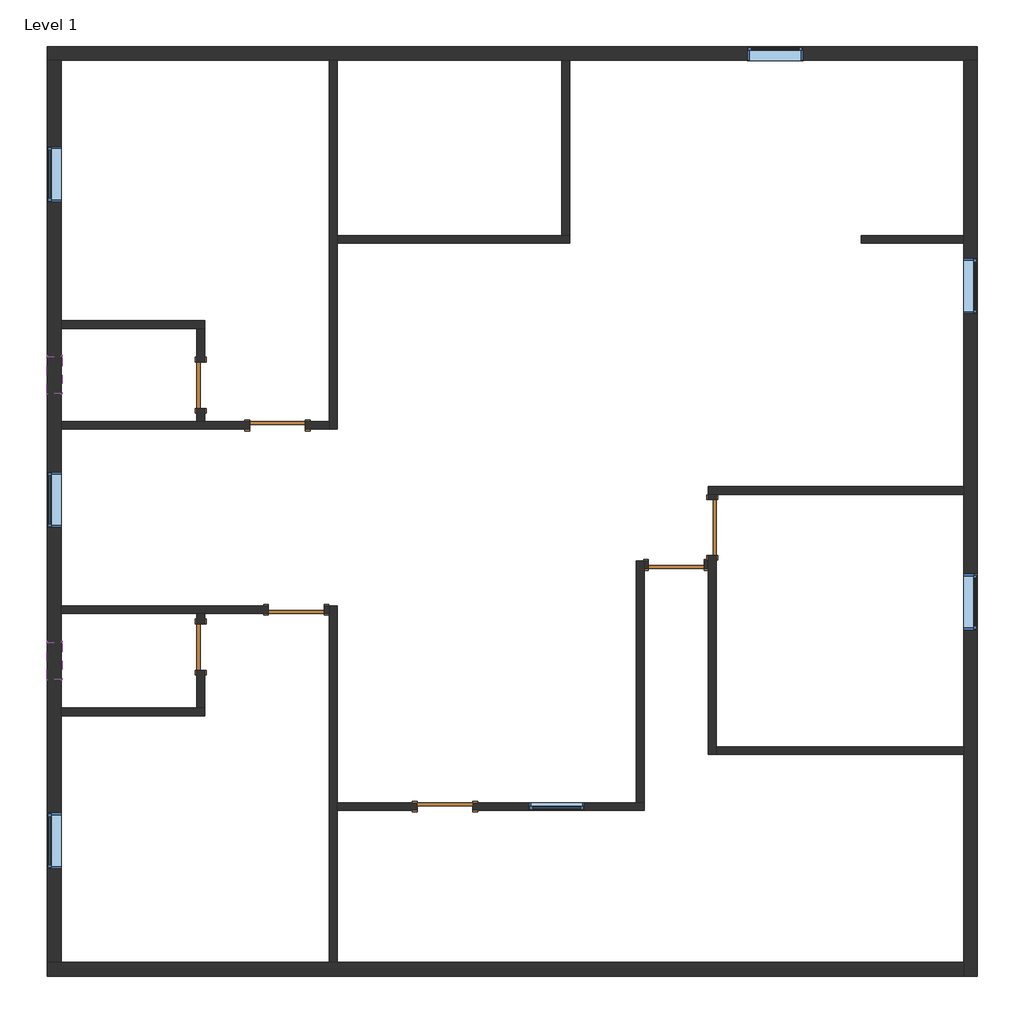
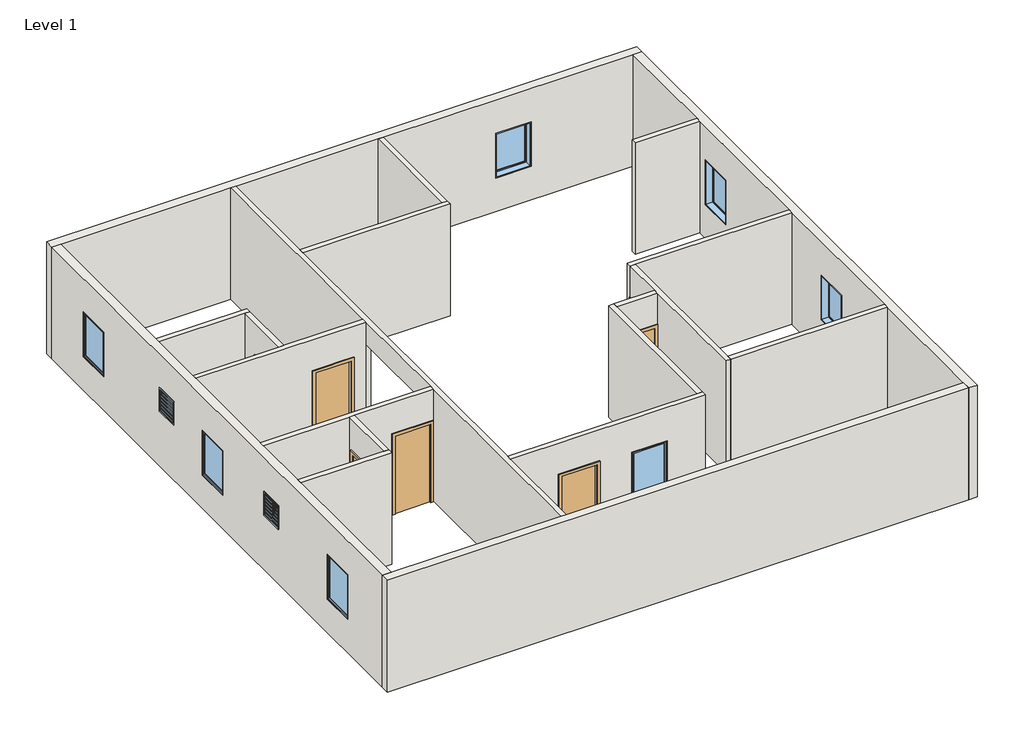
# One storey: 20 walls, 9 windows, 7 doors.
"""IFC4 building model written with IfcOpenShell, lengths in millimetres."""

from ifc_helpers import new_model, si_unit, frame, origin, origin_with_axes, place, context, project, spatial, polyline, outline, extrude, faceted_brep, transform, mapped, element, save
from components import door_4d6c7550, door_e36758a9, door_a1797ceb, door_a3eb833a, window_c1f32544, window_1bec9dad, window_f2d8fef0

model = new_model("IFC4")

# Units and contexts
model_context = context("Model", 3, world=origin())
ifc_project = project(units=[si_unit("LENGTHUNIT", "METRE", prefix="MILLI")], contexts=[model_context])

# Site, building, storey
site = spatial("IfcSite", under=ifc_project)
building = spatial("IfcBuilding", under=site)
storey = spatial("IfcBuildingStorey", under=building, Name="Level 1", Elevation=0.0)

# Doors
placement = place(None, origin())
door_shape = door_4d6c7550(model_context)
element("IfcDoor", 1, ObjectType="Single-Flush : 30\" x 84\"", at=placement, inside=storey, context=model_context, shape_type="MappedRepresentation", body=[
    mapped(door_shape, transform((-9496.7039913, -4083.9193327, 0.0), x_axis=(0.0, 1.0, 0.0), y_axis=(-1.0, 0.0, 0.0), z_axis=(0.0, 0.0, 1.0))),
])
door_2_shape = door_e36758a9(model_context)
element("IfcDoor", 2, ObjectType="Single-Flush : 30\" x 84\"", at=placement, inside=storey, context=model_context, shape_type="MappedRepresentation", body=[
    mapped(door_2_shape, transform((-9496.7039913, 208.6806673, 0.0), x_axis=(0.0, -1.0, 0.0), y_axis=(1.0, 0.0, 0.0), z_axis=(0.0, 0.0, 1.0))),
])
door_3_shape = door_a1797ceb(model_context)
element("IfcDoor", 3, ObjectType="Single-Flush : 36\" x 84\"", at=placement, inside=storey, context=model_context, shape_type="MappedRepresentation", body=[
    mapped(door_3_shape, transform((-8239.4039913, -451.7193327, 0.0), x_axis=(1.0, 0.0, 0.0), y_axis=(0.0, 1.0, 0.0), z_axis=(0.0, 0.0, 1.0))),
])
element("IfcDoor", 4, ObjectType="Single-Flush : 36\" x 84\"", at=placement, inside=storey, context=model_context, shape_type="MappedRepresentation", body=[
    mapped(door_3_shape, transform((-7934.6039913, -3474.3193327, 0.0), x_axis=(-1.0, 0.0, 0.0), y_axis=(0.0, -1.0, 0.0), z_axis=(0.0, 0.0, 1.0))),
])
element("IfcDoor", 5, ObjectType="Single-Flush : 36\" x 84\"", at=placement, inside=storey, context=model_context, shape_type="MappedRepresentation", body=[
    mapped(door_3_shape, transform((-1705.2539913, -2737.7193327, 0.0), x_axis=(-1.0, 0.0, 0.0), y_axis=(0.0, -1.0, 0.0), z_axis=(0.0, 0.0, 1.0))),
])
door_4_shape = door_a3eb833a(model_context)
element("IfcDoor", 6, ObjectType="Single-Flush : 36\" x 84\"", at=placement, inside=storey, context=model_context, shape_type="MappedRepresentation", body=[
    mapped(door_4_shape, transform((-1114.7039913, -2128.1193327, 0.0), x_axis=(0.0, 1.0, 0.0), y_axis=(-1.0, 0.0, 0.0), z_axis=(0.0, 0.0, 1.0))),
])
element("IfcDoor", 7, ObjectType="Single-Flush : 36\" x 84\"", at=placement, inside=storey, context=model_context, shape_type="MappedRepresentation", body=[
    mapped(door_4_shape, transform((-5496.2039913, -6700.1193327, 0.0), x_axis=(-1.0, 0.0, 0.0), y_axis=(0.0, -1.0, 0.0), z_axis=(0.0, 0.0, 1.0))),
])

# Walls
element("IfcWall", 8, ObjectType="Generic - 5\"", at=placement, inside=storey, context=model_context, shape_type="Brep", body=[
    faceted_brep([(-7261.5039913, 5529.9806673, 0.0), (-7261.5039913, 5529.9806673, 3048.0), (-7261.5039913, 2659.7806673, 3048.0), (-7261.5039913, 2532.7806673, 3048.0), (-7261.5039913, -6636.6193327, 3048.0), (-7261.5039913, -6763.6193327, 3048.0), (-7261.5039913, -9252.8193327, 3048.0), (-7261.5039913, -9252.8193327, 0.0), (-7261.5039913, -6763.6193327, 0.0), (-7261.5039913, -6636.6193327, 0.0), (-7261.5039913, -3410.8193327, 0.0), (-7261.5039913, -3410.8193327, 2438.4), (-7261.5039913, -515.2193327, 2438.4), (-7261.5039913, -515.2193327, 0.0), (-7261.5039913, 2532.7806673, 0.0), (-7261.5039913, 2659.7806673, 0.0), (-7388.5039913, 5529.9806673, 3048.0), (-7388.5039913, 5529.9806673, 0.0), (-7388.5039913, -388.2193327, 0.0), (-7388.5039913, -515.2193327, 0.0), (-7388.5039913, -515.2193327, 2438.4), (-7388.5039913, -3410.8193327, 2438.4), (-7388.5039913, -3410.8193327, 0.0), (-7388.5039913, -3537.8193327, 0.0), (-7388.5039913, -9252.8193327, 0.0), (-7388.5039913, -9252.8193327, 3048.0), (-7388.5039913, -3537.8193327, 3048.0), (-7388.5039913, -3410.8193327, 3048.0), (-7388.5039913, -515.2193327, 3048.0), (-7388.5039913, -388.2193327, 3048.0)], [[[0, 1, 2, 3, 4, 5, 6, 7, 8, 9, 10, 11, 12, 13, 14, 15]], [[16, 17, 18, 19, 20, 21, 22, 23, 24, 25, 26, 27, 28, 29]], [[7, 24, 23, 22, 10, 9, 8]], [[17, 0, 15, 14, 13, 19, 18]], [[6, 5, 4, 3, 2, 1, 16, 29, 28, 27, 26, 25]], [[7, 6, 25, 24]], [[1, 0, 17, 16]], [[11, 21, 20, 12]], [[21, 11, 10, 22]], [[12, 20, 19, 13]]]),
])
element("IfcWall", 9, ObjectType="Generic - 5\"", at=placement, inside=storey, context=model_context, shape_type="Brep", body=[
    faceted_brep([(-7261.5039913, 2532.7806673, 0.0), (-3451.5039913, 2532.7806673, 0.0), (-3451.5039913, 2532.7806673, 3048.0), (-7261.5039913, 2532.7806673, 3048.0), (-7261.5039913, 2659.7806673, 0.0), (-7261.5039913, 2659.7806673, 3048.0), (-3578.5039913, 2659.7806673, 3048.0), (-3451.5039913, 2659.7806673, 3048.0), (-3451.5039913, 2659.7806673, 0.0), (-3578.5039913, 2659.7806673, 0.0)], [[[0, 1, 2, 3]], [[4, 5, 6, 7, 8, 9]], [[1, 0, 4, 9, 8]], [[3, 2, 7, 6, 5]], [[0, 3, 5, 4]], [[2, 1, 8, 7]]]),
])
element("IfcWall", 10, ObjectType="Generic - 5\"", at=placement, inside=storey, context=model_context, shape_type="SweptSolid", body=[
    extrude(outline(polyline([(-3451.5039913, 5529.9806673), (-3451.5039913, 2659.7806673), (-3578.5039913, 2659.7806673), (-3578.5039913, 5529.9806673), (-3451.5039913, 5529.9806673)])), origin_with_axes(), (0.0, 0.0, 1.0), 3048.0),
])
element("IfcWall", 11, ObjectType="Generic - 5\"", at=placement, inside=storey, context=model_context, shape_type="SweptSolid", body=[
    extrude(outline(polyline([(1323.6960087, 2659.7806673), (3000.0960087, 2659.7806673), (3000.0960087, 2532.7806673), (1323.6960087, 2532.7806673), (1323.6960087, 2659.7806673)])), origin_with_axes(), (0.0, 0.0, 1.0), 3048.0),
])
element("IfcWall", 12, ObjectType="Generic - 5\"", at=placement, inside=storey, context=model_context, shape_type="SweptSolid", body=[
    extrude(outline(polyline([(0.0, -2232.3039913), (0.0, -2162.4539913), (2133.6, -2162.4539913), (2133.6, -1248.0539913), (0.0, -1248.0539913), (0.0, -1178.2039913), (3048.0, -1178.2039913), (3048.0, -2232.3039913), (0.0, -2232.3039913)])), frame((0.0, -2801.2193327, 0.0), z_axis=(0.0, 1.0, 0.0), x_axis=(0.0, 0.0, 1.0)), (0.0, 0.0, 1.0), 127.0),
])
element("IfcWall", 13, ObjectType="Generic - 5\"", at=placement, inside=storey, context=model_context, shape_type="Brep", body=[
    faceted_brep([(-1178.2039913, -1582.0193327, 0.0), (-1178.2039913, -1670.9193327, 0.0), (-1178.2039913, -1670.9193327, 2133.6), (-1178.2039913, -2585.3193327, 2133.6), (-1178.2039913, -2585.3193327, 0.0), (-1178.2039913, -2674.2193327, 0.0), (-1178.2039913, -2801.2193327, 0.0), (-1178.2039913, -5849.2193327, 0.0), (-1178.2039913, -5849.2193327, 3048.0), (-1178.2039913, -2801.2193327, 3048.0), (-1178.2039913, -2674.2193327, 3048.0), (-1178.2039913, -1582.0193327, 3048.0), (-1051.2039913, -1670.9193327, 2133.6), (-1051.2039913, -1670.9193327, 0.0), (-1051.2039913, -1582.0193327, 0.0), (-1051.2039913, -1582.0193327, 3048.0), (-1051.2039913, -5722.2193327, 3048.0), (-1051.2039913, -5849.2193327, 3048.0), (-1051.2039913, -5849.2193327, 0.0), (-1051.2039913, -5722.2193327, 0.0), (-1051.2039913, -2585.3193327, 0.0), (-1051.2039913, -2585.3193327, 2133.6)], [[[0, 1, 2, 3, 4, 5, 6, 7, 8, 9, 10, 11]], [[12, 13, 14, 15, 16, 17, 18, 19, 20, 21]], [[14, 13, 1, 0]], [[20, 19, 18, 7, 6, 5, 4]], [[11, 10, 9, 8, 17, 16, 15]], [[8, 7, 18, 17]], [[0, 11, 15, 14]], [[2, 1, 13, 12]], [[3, 2, 12, 21]], [[4, 3, 21, 20]]]),
])
element("IfcWall", 14, ObjectType="Generic - 5\"", at=placement, inside=storey, context=model_context, shape_type="SweptSolid", body=[
    extrude(outline(polyline([(3000.0960087, -5849.2193327), (-1051.2039913, -5849.2193327), (-1051.2039913, -5722.2193327), (3000.0960087, -5722.2193327), (3000.0960087, -5849.2193327)])), origin_with_axes(), (0.0, 0.0, 1.0), 3048.0),
])
element("IfcWall", 15, ObjectType="Generic - 5\"", at=placement, inside=storey, context=model_context, shape_type="Brep", body=[
    faceted_brep([(-7261.5039913, -6763.6193327, 0.0), (-5953.4039913, -6763.6193327, 0.0), (-5953.4039913, -6763.6193327, 2133.6), (-5039.0039913, -6763.6193327, 2133.6), (-5039.0039913, -6763.6193327, 0.0), (-2232.3039913, -6763.6193327, 0.0), (-2232.3039913, -6763.6193327, 3048.0), (-7261.5039913, -6763.6193327, 3048.0), (-4124.6039913, -6763.6193327, 2133.6), (-3210.2039913, -6763.6193327, 2133.6), (-3210.2039913, -6763.6193327, 914.4), (-4124.6039913, -6763.6193327, 914.4), (-5953.4039913, -6636.6193327, 2133.6), (-5953.4039913, -6636.6193327, 0.0), (-7261.5039913, -6636.6193327, 0.0), (-7261.5039913, -6636.6193327, 3048.0), (-2359.3039913, -6636.6193327, 3048.0), (-2232.3039913, -6636.6193327, 3048.0), (-2232.3039913, -6636.6193327, 0.0), (-2359.3039913, -6636.6193327, 0.0), (-5039.0039913, -6636.6193327, 0.0), (-5039.0039913, -6636.6193327, 2133.6), (-4124.6039913, -6636.6193327, 2133.6), (-4124.6039913, -6636.6193327, 914.4), (-3210.2039913, -6636.6193327, 914.4), (-3210.2039913, -6636.6193327, 2133.6)], [[[0, 1, 2, 3, 4, 5, 6, 7], [8, 9, 10, 11]], [[12, 13, 14, 15, 16, 17, 18, 19, 20, 21], [22, 23, 24, 25]], [[14, 13, 1, 0]], [[20, 19, 18, 5, 4]], [[7, 6, 17, 16, 15]], [[0, 7, 15, 14]], [[6, 5, 18, 17]], [[2, 1, 13, 12]], [[3, 2, 12, 21]], [[4, 3, 21, 20]], [[23, 22, 8, 11]], [[24, 23, 11, 10]], [[25, 24, 10, 9]], [[22, 25, 9, 8]]]),
])
element("IfcWall", 16, ObjectType="Generic - 5\"", at=placement, inside=storey, context=model_context, shape_type="Brep", body=[
    faceted_brep([(-2232.3039913, -6636.6193327, 0.0), (-2232.3039913, -2801.2193327, 0.0), (-2232.3039913, -2674.2193327, 0.0), (-2232.3039913, -2674.2193327, 3048.0), (-2232.3039913, -2801.2193327, 3048.0), (-2232.3039913, -6636.6193327, 3048.0), (-2359.3039913, -6636.6193327, 0.0), (-2359.3039913, -6636.6193327, 3048.0), (-2359.3039913, -2674.2193327, 3048.0), (-2359.3039913, -2674.2193327, 0.0)], [[[0, 1, 2, 3, 4, 5]], [[6, 7, 8, 9]], [[2, 1, 0, 6, 9]], [[5, 4, 3, 8, 7]], [[0, 5, 7, 6]], [[3, 2, 9, 8]]]),
])
element("IfcWall", 17, ObjectType="Generic - 5\"", at=placement, inside=storey, context=model_context, shape_type="Brep", body=[
    faceted_brep([(-11782.7039913, -5214.2193327, 0.0), (-9433.2039913, -5214.2193327, 0.0), (-9433.2039913, -5214.2193327, 3048.0), (-11782.7039913, -5214.2193327, 3048.0), (-11782.7039913, -5087.2193327, 0.0), (-11782.7039913, -5087.2193327, 3048.0), (-9560.2039913, -5087.2193327, 3048.0), (-9433.2039913, -5087.2193327, 3048.0), (-9433.2039913, -5087.2193327, 0.0), (-9560.2039913, -5087.2193327, 0.0)], [[[0, 1, 2, 3]], [[4, 5, 6, 7, 8, 9]], [[1, 0, 4, 9, 8]], [[3, 2, 7, 6, 5]], [[0, 3, 5, 4]], [[2, 1, 8, 7]]]),
])
element("IfcWall", 18, ObjectType="Generic - 5\"", at=placement, inside=storey, context=model_context, shape_type="SweptSolid", body=[
    extrude(outline(polyline([(-3537.8193327, 0.0), (-3702.9193327, 0.0), (-3702.9193327, 2133.6), (-4464.9193327, 2133.6), (-4464.9193327, 0.0), (-5087.2193327, 0.0), (-5087.2193327, 3048.0), (-3537.8193327, 3048.0), (-3537.8193327, 0.0)])), frame((-9560.2039913, 0.0, 0.0), z_axis=(1.0, 0.0, 0.0), x_axis=(0.0, 1.0, 0.0)), (0.0, 0.0, 1.0), 127.0),
])
element("IfcWall", 19, ObjectType="Generic - 5\"", at=placement, inside=storey, context=model_context, shape_type="Brep", body=[
    faceted_brep([(-8391.8039913, -3410.8193327, 2133.6), (-8391.8039913, -3410.8193327, 0.0), (-11782.7039913, -3410.8193327, 0.0), (-11782.7039913, -3410.8193327, 3048.0), (-7388.5039913, -3410.8193327, 3048.0), (-7388.5039913, -3410.8193327, 2438.4), (-7388.5039913, -3410.8193327, 0.0), (-7477.4039913, -3410.8193327, 0.0), (-7477.4039913, -3410.8193327, 2133.6), (-11782.7039913, -3537.8193327, 0.0), (-9560.2039913, -3537.8193327, 0.0), (-9433.2039913, -3537.8193327, 0.0), (-8391.8039913, -3537.8193327, 0.0), (-8391.8039913, -3537.8193327, 2133.6), (-7477.4039913, -3537.8193327, 2133.6), (-7477.4039913, -3537.8193327, 0.0), (-7388.5039913, -3537.8193327, 0.0), (-7388.5039913, -3537.8193327, 3048.0), (-9433.2039913, -3537.8193327, 3048.0), (-9560.2039913, -3537.8193327, 3048.0), (-11782.7039913, -3537.8193327, 3048.0)], [[[0, 1, 2, 3, 4, 5, 6, 7, 8]], [[9, 10, 11, 12, 13, 14, 15, 16, 17, 18, 19, 20]], [[7, 6, 16, 15]], [[2, 1, 12, 11, 10, 9]], [[4, 3, 20, 19, 18, 17]], [[3, 2, 9, 20]], [[6, 5, 4, 17, 16]], [[13, 12, 1, 0]], [[14, 13, 0, 8]], [[15, 14, 8, 7]]]),
])
element("IfcWall", 20, ObjectType="Generic - 5\"", at=placement, inside=storey, context=model_context, shape_type="Brep", body=[
    faceted_brep([(-7388.5039913, -388.2193327, 0.0), (-7782.2039913, -388.2193327, 0.0), (-7782.2039913, -388.2193327, 2133.6), (-8696.6039913, -388.2193327, 2133.6), (-8696.6039913, -388.2193327, 0.0), (-9433.2039913, -388.2193327, 0.0), (-9560.2039913, -388.2193327, 0.0), (-11782.7039913, -388.2193327, 0.0), (-11782.7039913, -388.2193327, 3048.0), (-9560.2039913, -388.2193327, 3048.0), (-9433.2039913, -388.2193327, 3048.0), (-7388.5039913, -388.2193327, 3048.0), (-7782.2039913, -515.2193327, 2133.6), (-7782.2039913, -515.2193327, 0.0), (-7388.5039913, -515.2193327, 0.0), (-7388.5039913, -515.2193327, 2438.4), (-7388.5039913, -515.2193327, 3048.0), (-11782.7039913, -515.2193327, 3048.0), (-11782.7039913, -515.2193327, 0.0), (-8696.6039913, -515.2193327, 0.0), (-8696.6039913, -515.2193327, 2133.6)], [[[0, 1, 2, 3, 4, 5, 6, 7, 8, 9, 10, 11]], [[12, 13, 14, 15, 16, 17, 18, 19, 20]], [[19, 18, 7, 6, 5, 4]], [[14, 13, 1, 0]], [[11, 10, 9, 8, 17, 16]], [[8, 7, 18, 17]], [[0, 11, 16, 15, 14]], [[2, 1, 13, 12]], [[3, 2, 12, 20]], [[4, 3, 20, 19]]]),
])
element("IfcWall", 21, ObjectType="Generic - 5\"", at=placement, inside=storey, context=model_context, shape_type="Brep", body=[
    faceted_brep([(-9433.2039913, 1262.7806673, 0.0), (-11782.7039913, 1262.7806673, 0.0), (-11782.7039913, 1262.7806673, 3048.0), (-9433.2039913, 1262.7806673, 3048.0), (-9433.2039913, 1135.7806673, 0.0), (-9433.2039913, 1135.7806673, 3048.0), (-9560.2039913, 1135.7806673, 3048.0), (-11782.7039913, 1135.7806673, 3048.0), (-11782.7039913, 1135.7806673, 0.0), (-9560.2039913, 1135.7806673, 0.0)], [[[0, 1, 2, 3]], [[4, 5, 6, 7, 8, 9]], [[1, 0, 4, 9, 8]], [[3, 2, 7, 6, 5]], [[2, 1, 8, 7]], [[0, 3, 5, 4]]]),
])
element("IfcWall", 22, ObjectType="Generic - 5\"", at=placement, inside=storey, context=model_context, shape_type="SweptSolid", body=[
    extrude(outline(polyline([(-172.3193327, 2133.6), (-172.3193327, 0.0), (-388.2193327, 0.0), (-388.2193327, 3048.0), (1135.7806673, 3048.0), (1135.7806673, 0.0), (589.6806673, 0.0), (589.6806673, 2133.6), (-172.3193327, 2133.6)])), frame((-9560.2039913, 0.0, 0.0), z_axis=(1.0, 0.0, 0.0), x_axis=(0.0, 1.0, 0.0)), (0.0, 0.0, 1.0), 127.0),
])
element("IfcWall", 23, ObjectType="Generic - 5\"", at=placement, inside=storey, context=model_context, shape_type="Brep", body=[
    faceted_brep([(3000.0960087, -1455.0193327, 0.0), (-1178.2039913, -1455.0193327, 0.0), (-1178.2039913, -1455.0193327, 3048.0), (3000.0960087, -1455.0193327, 3048.0), (3000.0960087, -1582.0193327, 0.0), (3000.0960087, -1582.0193327, 3048.0), (-1051.2039913, -1582.0193327, 3048.0), (-1178.2039913, -1582.0193327, 3048.0), (-1178.2039913, -1582.0193327, 0.0), (-1051.2039913, -1582.0193327, 0.0)], [[[0, 1, 2, 3]], [[4, 5, 6, 7, 8, 9]], [[1, 0, 4, 9, 8]], [[3, 2, 7, 6, 5]], [[0, 3, 5, 4]], [[2, 1, 8, 7]]]),
])
element("IfcWall", 24, ObjectType="Generic - 9\"", at=placement, inside=storey, context=model_context, shape_type="Brep", body=[
    faceted_brep([(-12011.3039913, 5529.9806673, 0.0), (-11782.7039913, 5529.9806673, 0.0), (-7388.5039913, 5529.9806673, 0.0), (-7261.5039913, 5529.9806673, 0.0), (-3578.5039913, 5529.9806673, 0.0), (-3451.5039913, 5529.9806673, 0.0), (3000.0960087, 5529.9806673, 0.0), (3228.6960087, 5529.9806673, 0.0), (3228.6960087, 5529.9806673, 3048.0), (3000.0960087, 5529.9806673, 3048.0), (-3451.5039913, 5529.9806673, 3048.0), (-3578.5039913, 5529.9806673, 3048.0), (-7261.5039913, 5529.9806673, 3048.0), (-7388.5039913, 5529.9806673, 3048.0), (-11782.7039913, 5529.9806673, 3048.0), (-12011.3039913, 5529.9806673, 3048.0), (371.1960087, 5529.9806673, 2133.6), (371.1960087, 5529.9806673, 914.4), (-543.2039913, 5529.9806673, 914.4), (-543.2039913, 5529.9806673, 2133.6), (-12011.3039913, 5758.5806673, 0.0), (-12011.3039913, 5758.5806673, 3048.0), (3228.6960087, 5758.5806673, 3048.0), (3228.6960087, 5758.5806673, 0.0), (371.1960087, 5758.5806673, 2133.6), (-543.2039913, 5758.5806673, 2133.6), (-543.2039913, 5758.5806673, 914.4), (371.1960087, 5758.5806673, 914.4)], [[[0, 1, 2, 3, 4, 5, 6, 7, 8, 9, 10, 11, 12, 13, 14, 15], [16, 17, 18, 19]], [[20, 21, 22, 23], [24, 25, 26, 27]], [[7, 6, 5, 4, 3, 2, 1, 0, 20, 23]], [[15, 14, 13, 12, 11, 10, 9, 8, 22, 21]], [[8, 7, 23, 22]], [[0, 15, 21, 20]], [[17, 16, 24, 27]], [[18, 17, 27, 26]], [[19, 18, 26, 25]], [[16, 19, 25, 24]]]),
])
element("IfcWall", 25, ObjectType="Generic - 9\"", at=placement, inside=storey, context=model_context, shape_type="Brep", body=[
    faceted_brep([(3000.0960087, 5529.9806673, 0.0), (3000.0960087, 2659.7806673, 0.0), (3000.0960087, 2532.7806673, 0.0), (3000.0960087, -1455.0193327, 0.0), (3000.0960087, -1582.0193327, 0.0), (3000.0960087, -5722.2193327, 0.0), (3000.0960087, -5849.2193327, 0.0), (3000.0960087, -9252.8193327, 0.0), (3000.0960087, -9481.4193327, 0.0), (3000.0960087, -9481.4193327, 3048.0), (3000.0960087, -9252.8193327, 3048.0), (3000.0960087, -5849.2193327, 3048.0), (3000.0960087, -5722.2193327, 3048.0), (3000.0960087, -1582.0193327, 3048.0), (3000.0960087, -1455.0193327, 3048.0), (3000.0960087, 2532.7806673, 3048.0), (3000.0960087, 2659.7806673, 3048.0), (3000.0960087, 5529.9806673, 3048.0), (3000.0960087, -3804.5193327, 2133.6), (3000.0960087, -3804.5193327, 914.4), (3000.0960087, -2890.1193327, 914.4), (3000.0960087, -2890.1193327, 2133.6), (3000.0960087, 1377.0806673, 2133.6), (3000.0960087, 1377.0806673, 914.4), (3000.0960087, 2291.4806673, 914.4), (3000.0960087, 2291.4806673, 2133.6), (3228.6960087, 5529.9806673, 0.0), (3228.6960087, 5529.9806673, 3048.0), (3228.6960087, -9481.4193327, 3048.0), (3228.6960087, -9481.4193327, 0.0), (3228.6960087, -3804.5193327, 2133.6), (3228.6960087, -2890.1193327, 2133.6), (3228.6960087, -2890.1193327, 914.4), (3228.6960087, -3804.5193327, 914.4), (3228.6960087, 1377.0806673, 2133.6), (3228.6960087, 2291.4806673, 2133.6), (3228.6960087, 2291.4806673, 914.4), (3228.6960087, 1377.0806673, 914.4)], [[[0, 1, 2, 3, 4, 5, 6, 7, 8, 9, 10, 11, 12, 13, 14, 15, 16, 17], [18, 19, 20, 21], [22, 23, 24, 25]], [[26, 27, 28, 29], [30, 31, 32, 33], [34, 35, 36, 37]], [[8, 7, 6, 5, 4, 3, 2, 1, 0, 26, 29]], [[17, 16, 15, 14, 13, 12, 11, 10, 9, 28, 27]], [[0, 17, 27, 26]], [[9, 8, 29, 28]], [[19, 18, 30, 33]], [[20, 19, 33, 32]], [[21, 20, 32, 31]], [[18, 21, 31, 30]], [[23, 22, 34, 37]], [[24, 23, 37, 36]], [[25, 24, 36, 35]], [[22, 25, 35, 34]]]),
])
element("IfcWall", 26, ObjectType="Generic - 9\"", at=placement, inside=storey, context=model_context, shape_type="Brep", body=[
    faceted_brep([(3000.0960087, -9252.8193327, 0.0), (-7261.5039913, -9252.8193327, 0.0), (-7388.5039913, -9252.8193327, 0.0), (-11782.7039913, -9252.8193327, 0.0), (-12011.3039913, -9252.8193327, 0.0), (-12011.3039913, -9252.8193327, 3048.0), (-11782.7039913, -9252.8193327, 3048.0), (-7388.5039913, -9252.8193327, 3048.0), (-7261.5039913, -9252.8193327, 3048.0), (3000.0960087, -9252.8193327, 3048.0), (3000.0960087, -9481.4193327, 0.0), (3000.0960087, -9481.4193327, 3048.0), (-12011.3039913, -9481.4193327, 3048.0), (-12011.3039913, -9481.4193327, 0.0)], [[[0, 1, 2, 3, 4, 5, 6, 7, 8, 9]], [[10, 11, 12, 13]], [[4, 3, 2, 1, 0, 10, 13]], [[9, 8, 7, 6, 5, 12, 11]], [[0, 9, 11, 10]], [[5, 4, 13, 12]]]),
])
element("IfcWall", 27, ObjectType="Generic - 9\"", at=placement, inside=storey, context=model_context, shape_type="Brep", body=[
    faceted_brep([(-11782.7039913, -9252.8193327, 0.0), (-11782.7039913, -5214.2193327, 0.0), (-11782.7039913, -5087.2193327, 0.0), (-11782.7039913, -3537.8193327, 0.0), (-11782.7039913, -3410.8193327, 0.0), (-11782.7039913, -515.2193327, 0.0), (-11782.7039913, -388.2193327, 0.0), (-11782.7039913, 1135.7806673, 0.0), (-11782.7039913, 1262.7806673, 0.0), (-11782.7039913, 5529.9806673, 0.0), (-11782.7039913, 5529.9806673, 3048.0), (-11782.7039913, 1262.7806673, 3048.0), (-11782.7039913, 1135.7806673, 3048.0), (-11782.7039913, -388.2193327, 3048.0), (-11782.7039913, -515.2193327, 3048.0), (-11782.7039913, -3410.8193327, 3048.0), (-11782.7039913, -3537.8193327, 3048.0), (-11782.7039913, -5087.2193327, 3048.0), (-11782.7039913, -5214.2193327, 3048.0), (-11782.7039913, -9252.8193327, 3048.0), (-11782.7039913, 4120.2806673, 2133.6), (-11782.7039913, 4120.2806673, 914.4), (-11782.7039913, 3205.8806673, 914.4), (-11782.7039913, 3205.8806673, 2133.6), (-11782.7039913, -6801.7193327, 2133.6), (-11782.7039913, -6801.7193327, 914.4), (-11782.7039913, -7716.1193327, 914.4), (-11782.7039913, -7716.1193327, 2133.6), (-11782.7039913, -1213.7193327, 2133.6), (-11782.7039913, -1213.7193327, 914.4), (-11782.7039913, -2128.1193327, 914.4), (-11782.7039913, -2128.1193327, 2133.6), (-11782.7039913, 68.9806673, 2133.6), (-11782.7039913, 678.5806673, 2133.6), (-11782.7039913, 678.5806673, 1524.0), (-11782.7039913, 68.9806673, 1524.0), (-11782.7039913, -4617.3193327, 2133.6), (-11782.7039913, -4007.7193327, 2133.6), (-11782.7039913, -4007.7193327, 1524.0), (-11782.7039913, -4617.3193327, 1524.0), (-12011.3039913, -9252.8193327, 0.0), (-12011.3039913, -9252.8193327, 3048.0), (-12011.3039913, 5529.9806673, 3048.0), (-12011.3039913, 5529.9806673, 0.0), (-12011.3039913, 4120.2806673, 2133.6), (-12011.3039913, 3205.8806673, 2133.6), (-12011.3039913, 3205.8806673, 914.4), (-12011.3039913, 4120.2806673, 914.4), (-12011.3039913, -6801.7193327, 2133.6), (-12011.3039913, -7716.1193327, 2133.6), (-12011.3039913, -7716.1193327, 914.4), (-12011.3039913, -6801.7193327, 914.4), (-12011.3039913, -1213.7193327, 2133.6), (-12011.3039913, -2128.1193327, 2133.6), (-12011.3039913, -2128.1193327, 914.4), (-12011.3039913, -1213.7193327, 914.4), (-12011.3039913, 68.9806673, 2133.6), (-12011.3039913, 68.9806673, 1524.0), (-12011.3039913, 678.5806673, 1524.0), (-12011.3039913, 678.5806673, 2133.6), (-12011.3039913, -4617.3193327, 2133.6), (-12011.3039913, -4617.3193327, 1524.0), (-12011.3039913, -4007.7193327, 1524.0), (-12011.3039913, -4007.7193327, 2133.6)], [[[0, 1, 2, 3, 4, 5, 6, 7, 8, 9, 10, 11, 12, 13, 14, 15, 16, 17, 18, 19], [20, 21, 22, 23], [24, 25, 26, 27], [28, 29, 30, 31], [32, 33, 34, 35], [36, 37, 38, 39]], [[40, 41, 42, 43], [44, 45, 46, 47], [48, 49, 50, 51], [52, 53, 54, 55], [56, 57, 58, 59], [60, 61, 62, 63]], [[9, 8, 7, 6, 5, 4, 3, 2, 1, 0, 40, 43]], [[19, 18, 17, 16, 15, 14, 13, 12, 11, 10, 42, 41]], [[0, 19, 41, 40]], [[10, 9, 43, 42]], [[21, 20, 44, 47]], [[22, 21, 47, 46]], [[23, 22, 46, 45]], [[20, 23, 45, 44]], [[25, 24, 48, 51]], [[26, 25, 51, 50]], [[27, 26, 50, 49]], [[24, 27, 49, 48]], [[29, 28, 52, 55]], [[30, 29, 55, 54]], [[31, 30, 54, 53]], [[28, 31, 53, 52]], [[57, 56, 32, 35]], [[58, 57, 35, 34]], [[59, 58, 34, 33]], [[56, 59, 33, 32]], [[61, 60, 36, 39]], [[62, 61, 39, 38]], [[63, 62, 38, 37]], [[60, 63, 37, 36]]]),
])

# Windows
window_shape = window_c1f32544(model_context)
element("IfcWindow", 28, ObjectType="Fixed : 36\" x 48\"", at=placement, inside=storey, context=model_context, shape_type="MappedRepresentation", body=[
    mapped(window_shape, transform((-11897.0039913, 3701.1806673, 0.0), x_axis=(0.0, 1.0, 0.0), y_axis=(-1.0, 0.0, 0.0), z_axis=(0.0, 0.0, 1.0))),
])
element("IfcWindow", 29, ObjectType="Fixed : 36\" x 48\"", at=placement, inside=storey, context=model_context, shape_type="MappedRepresentation", body=[
    mapped(window_shape, transform((-11897.0039913, -7220.8193327, 0.0), x_axis=(0.0, 1.0, 0.0), y_axis=(-1.0, 0.0, 0.0), z_axis=(0.0, 0.0, 1.0))),
])
element("IfcWindow", 30, ObjectType="Fixed : 36\" x 48\"", at=placement, inside=storey, context=model_context, shape_type="MappedRepresentation", body=[
    mapped(window_shape, transform((3114.3960087, -3385.4193327, 0.0), x_axis=(0.0, -1.0, 0.0), y_axis=(1.0, 0.0, 0.0), z_axis=(0.0, 0.0, 1.0))),
])
element("IfcWindow", 31, ObjectType="Fixed : 36\" x 48\"", at=placement, inside=storey, context=model_context, shape_type="MappedRepresentation", body=[
    mapped(window_shape, transform((3114.3960087, 1796.1806673, 0.0), x_axis=(0.0, -1.0, 0.0), y_axis=(1.0, 0.0, 0.0), z_axis=(0.0, 0.0, 1.0))),
])
element("IfcWindow", 32, ObjectType="Fixed : 36\" x 48\"", at=placement, inside=storey, context=model_context, shape_type="MappedRepresentation", body=[
    mapped(window_shape, transform((-47.9039913, 5644.2806673, 0.0), x_axis=(1.0, 0.0, 0.0), y_axis=(0.0, 1.0, 0.0), z_axis=(0.0, 0.0, 1.0))),
])
element("IfcWindow", 33, ObjectType="Fixed : 36\" x 48\"", at=placement, inside=storey, context=model_context, shape_type="MappedRepresentation", body=[
    mapped(window_shape, transform((-11897.0039913, -1632.8193327, 0.0), x_axis=(0.0, 1.0, 0.0), y_axis=(-1.0, 0.0, 0.0), z_axis=(0.0, 0.0, 1.0))),
])
window_2_shape = window_1bec9dad(model_context)
element("IfcWindow", 34, ObjectType="Fixed : 36\" x 48\"", at=placement, inside=storey, context=model_context, shape_type="MappedRepresentation", body=[
    mapped(window_2_shape, transform((-3705.5039913, -6700.1193327, 0.0), x_axis=(-1.0, 0.0, 0.0), y_axis=(0.0, -1.0, 0.0), z_axis=(0.0, 0.0, 1.0))),
])
window_3_shape = window_f2d8fef0(model_context)
element("IfcWindow", 35, ObjectType="Window-Louvers : 24\" x 24\"", at=placement, inside=storey, context=model_context, shape_type="MappedRepresentation", body=[
    mapped(window_3_shape, transform((-11903.3539913, 373.7806673, 609.6), x_axis=(0.0, 1.0, 0.0), y_axis=(-1.0, 0.0, 0.0), z_axis=(0.0, 0.0, 1.0))),
])
element("IfcWindow", 36, ObjectType="Window-Louvers : 24\" x 24\"", at=placement, inside=storey, context=model_context, shape_type="MappedRepresentation", body=[
    mapped(window_3_shape, transform((-11903.3539913, -4312.5193327, 609.6), x_axis=(0.0, 1.0, 0.0), y_axis=(-1.0, 0.0, 0.0), z_axis=(0.0, 0.0, 1.0))),
])

save(model, "model.ifc")

# Revit data of these elements
# Type "Single-Flush : 30\" x 84\""
#   Type Mark = "4"
#   Construction Type Id = "MDOOR"
#   Assembly Code = "C1020"
#   Analytic Construction = "Metal"
#   Thickness = 0' - 2"
#   Heat Transfer Coefficient (U) = 0.651978 BTU/(h·ft²·°F)
#   Height = 7' - 0"
#   Trim Projection Ext = 0' - 1"
#   Trim Projection Int = 0' - 1"
#   Trim Width = 0' - 3"
#   Width = 2' - 6"
#   Define Thermal Properties by = 1
#   Define Thermal Properties by = 1
#   Door Material = Door - Panel
#   Frame Material = Door - Frame
#   Visual Light Transmittance = 0
#   Solar Heat Gain Coefficient = 0
#   Function = (empty or 0)
#   Wall Closure = (empty or 0)
# Type "Single-Flush : 36\" x 84\""
#   Type Mark = "1"
#   Construction Type Id = "MDOOR"
#   Assembly Code = "C1020"
#   Analytic Construction = "Metal"
#   Thickness = 0' - 2"
#   Heat Transfer Coefficient (U) = 0.651978 BTU/(h·ft²·°F)
#   Height = 7' - 0"
#   Trim Projection Ext = 0' - 1"
#   Trim Projection Int = 0' - 1"
#   Trim Width = 0' - 3"
#   Width = 3' - 0"
#   Define Thermal Properties by = 1
#   Define Thermal Properties by = 1
#   Door Material = Door - Panel
#   Frame Material = Door - Frame
#   Visual Light Transmittance = 0
#   Solar Heat Gain Coefficient = 0
#   Function = (empty or 0)
#   Wall Closure = (empty or 0)
# Type "Generic - 5\""
#   Assembly Code = "B2010"
#   Layers, outside or top first: 0' - 5" no material (function 1)
# Type "Generic - 9\""
#   Assembly Code = "B2010"
#   Layers, outside or top first: 0' - 9" no material (function 1)
# Type "Fixed : 36\" x 48\""
#   Type Mark = "W1"
#   Construction Type Id = "GSP4R"
#   Assembly Code = "B2020100"
#   Analytic Construction = "1/8 in Pilkington single glazing"
#   Visual Light Transmittance = 0.9
#   Solar Heat Gain Coefficient = 0.78
#   Heat Transfer Coefficient (U) = 0.6496 BTU/(h·ft²·°F)
#   Height = 4' - 0"
#   Default Sill Height = 3' - 0"
#   Width = 3' - 0"
#   Window Inset = 0' - 0 3/4"
#   Define Thermal Properties by = 1
#   Define Thermal Properties by = 1
#   Glass Pane Material = Glass
#   Sash Material = Sash
#   Wall Closure = (empty or 0)
# Type "Window-Louvers : 24\" x 24\""
#   Type Mark = "V1"
#   Construction Type Id = "GSP4R"
#   Assembly Code = "B20"
#   Analytic Construction = "1/8 in Pilkington single glazing"
#   Visual Light Transmittance = 0.9
#   Thermal Resistance (R) = 1.53941 (h·ft²·°F)/BTU
#   Solar Heat Gain Coefficient = 0.78
#   Max Height = 1' - 11.74264"
#   Height = 2' - 0"
#   Heat Transfer Coefficient (U) = 0.6496 BTU/(h·ft²·°F)
#   Blade Width [instance default] = 1' - 10 1/2"
#   Blade Vertical Thickness = 0' - 0.35355"
#   Blade Thickness = 0' - 0 1/4"
#   Blade Spacing = 0' - 1 1/2"
#   Blade Height = 0' - 1.85355"
#   Blade Depth = 0' - 3"
#   Blade Angle = 45.00°
#   Default Sill Height = 3' - 0"
#   Trim Projection_Exterior = 0' - 0 1/2"
#   Trim Projection_Interior = 0' - 0 1/2"
#   Trim Width_Exterior = 0' - 1 1/2"
#   Trim Width_Interior = 0' - 1 1/2"
#   Width = 2' - 0"
#   Max Blade Count = 12
#   Define Thermal Properties by = 1
#   Blade Count = 12
#   Frame Material = Birch
#   Louver Material = Birch
#   Trim Exterior Material = Birch
#   Trim Interior Material = Birch
#   Wall Closure = (empty or 0)
# Elements 1, 2 (IfcDoor, "Single-Flush : 30\" x 84\"")
#   Phase Created = New Construction
#   Materials on its faces: "Door - Frame", "Door - Panel"
# Elements 3, 4, 5, 6, 7 (IfcDoor, "Single-Flush : 36\" x 84\"")
#   Phase Created = New Construction
#   Materials on its faces: "Door - Frame", "Door - Panel"
# Elements 8, 9, 10, 11, 12, 13, 14, 15, 16, 17, 18, 19, 20, 21, 22, 23 (IfcWall, "Generic - 5\"")
#   Top Offset = 0' - 0"
#   Base Offset = 0' - 0"
#   wall height = 10' - 0"
#   Phase Created = New Construction
#   Base Constraint = Level 1
#   Top Constraint = Level 2
#   Materials on its faces: "Default Wall"
# Elements 24, 25, 26, 27 (IfcWall, "Generic - 9\"")
#   Top Offset = 0' - 0"
#   Base Offset = 0' - 0"
#   wall height = 10' - 0"
#   Phase Created = New Construction
#   Base Constraint = Level 1
#   Top Constraint = Level 2
#   Materials on its faces: "Default Wall"
# Element 28 (IfcWindow, "Fixed : 36\" x 48\"")
#   Mark = "1"
#   Phase Created = New Construction
#   Materials on its faces: "Sash", "Glass"
# Element 29 (IfcWindow, "Fixed : 36\" x 48\"")
#   Mark = "2"
#   Phase Created = New Construction
#   Materials on its faces: "Sash", "Glass"
# Element 30 (IfcWindow, "Fixed : 36\" x 48\"")
#   Mark = "4"
#   Phase Created = New Construction
#   Materials on its faces: "Sash", "Glass"
# Element 31 (IfcWindow, "Fixed : 36\" x 48\"")
#   Mark = "5"
#   Phase Created = New Construction
#   Materials on its faces: "Sash", "Glass"
# Element 32 (IfcWindow, "Fixed : 36\" x 48\"")
#   Mark = "6"
#   Phase Created = New Construction
#   Materials on its faces: "Sash", "Glass"
# Element 33 (IfcWindow, "Fixed : 36\" x 48\"")
#   Mark = "7"
#   Phase Created = New Construction
#   Materials on its faces: "Sash", "Glass"
# Element 34 (IfcWindow, "Fixed : 36\" x 48\"")
#   Mark = "3"
#   Phase Created = New Construction
#   Materials on its faces: "Sash", "Glass"
# Element 35 (IfcWindow, "Window-Louvers : 24\" x 24\"")
#   Mark = "8"
#   Blade Width = 1' - 10 1/2"
#   Phase Created = New Construction
#   Materials on its faces: "Birch"
# Element 36 (IfcWindow, "Window-Louvers : 24\" x 24\"")
#   Mark = "9"
#   Blade Width = 1' - 10 1/2"
#   Phase Created = New Construction
#   Materials on its faces: "Birch"
# Materials
#   "Door - Panel": class "Wood", colour RGB 210 159 95, transparency 0, Cost = 0
#   "Door - Frame": colour RGB 118 70 51, transparency 0, Cost = 0
#   "Glass": class "Glass", colour RGB 0 128 192, transparency 0.75, Description = "Soda Lime Glass", Cost = 0
#   "Sash": class "Wood", colour RGB 224 178 126, transparency 0, Cost = 0
#   "Birch": class "Wood", colour RGB 224 178 126, transparency 0, Description = "Betula Alleghaniensis", Cost = 0
#   "Default Wall": colour RGB 128 128 128, transparency 0, Cost = 0
# Area at (-9501.861, -6788.825) mm, upper offset 10' - 0", lower offset 0' - 0"
#   Number = "5"
#   Name = "Area"
# Area at (-4165.808, 865.922) mm, upper offset 10' - 0", lower offset 0' - 0"
#   Number = "6"
#   Name = "Area"
# Area at (-5544.368, 4043.256) mm, upper offset 10' - 0", lower offset 0' - 0"
#   Number = "7"
#   Name = "Area"
# Area at (756.344, 378.604) mm, upper offset 0' - 0", lower offset 0' - 0"
#   Number = "8"
#   Name = "Area"
# Area at (1128.367, -3617.061) mm, upper offset 0' - 0", lower offset 0' - 0"
#   Number = "9"
#   Name = "Area"
# Area at (0, 4589.064) mm, upper offset 0' - 0", lower offset 0' - 0"
#   Number = "10"
#   Name = "Area"
# Area at (-4844.312, -3031.24) mm, upper offset 0' - 0", lower offset 0' - 0"
#   Number = "11"
#   Name = "Area"
# Room at (-514.743, 4105.555) mm, phase "New Construction", upper level "Level 1", upper offset 10' - 0", lower offset 0' - 0"
#   Number = "1"
#   Name = "Utility"
# Room at (-5259.391, 4105.555) mm, phase "New Construction", upper level "Level 1", upper offset 10' - 0", lower offset 0' - 0"
#   Number = "2"
#   Name = "Balcony"
# Room at (-9010.101, 4105.555) mm, phase "New Construction", upper level "Level 1", upper offset 10' - 0", lower offset 0' - 0"
#   Number = "3"
#   Name = "Room 1"
# Room at (-10838.901, 350.488) mm, phase "New Construction", upper level "Level 1", upper offset 10' - 0", lower offset 0' - 0"
#   Number = "4"
#   Name = "Toilet 1"
# Room at (-10611.42, -4256.828) mm, phase "New Construction", upper level "Level 1", upper offset 10' - 0", lower offset 0' - 0"
#   Number = "5"
#   Name = "Toilet 2"
# Room at (-9716.811, -7044.793) mm, phase "New Construction", upper level "Level 1", upper offset 10' - 0", lower offset 0' - 0"
#   Number = "6"
#   Name = "Room 2"
# Room at (619.442, -3821.027) mm, phase "New Construction", upper level "Level 1", upper offset 10' - 0", lower offset 0' - 0"
#   Number = "7"
#   Name = "Room 3"
# Room at (-4393.41, 788.834) mm, phase "New Construction", upper level "Level 1", upper offset 10' - 0", lower offset 0' - 0"
#   Number = "8"
#   Name = "Dining"
# Room at (-4393.41, -2561.835) mm, phase "New Construction", upper level "Level 1", upper offset 10' - 0", lower offset 0' - 0"
#   Number = "9"
#   Name = "HALL"
# Room at (2162.831, 350.488) mm, phase "New Construction", upper level "Level 1", upper offset 10' - 0", lower offset 0' - 0"
#   Number = "10"
#   Name = "Kitchen"
# Area at (-9336.292, 3129.677) mm, upper offset 10' - 0", lower offset 0' - 0"
#   Number = "1"
#   Name = "Area"
# Area at (-10762.821, 378.604) mm, upper offset 10' - 0", lower offset 0' - 0"
#   Number = "2"
#   Name = "Area"
# Area at (-10050.186, -1909.329) mm, upper offset 10' - 0", lower offset 0' - 0"
#   Number = "3"
#   Name = "Area"
# Area at (-10722.071, -4386.21) mm, upper offset 10' - 0", lower offset 0' - 0"
#   Number = "4"
#   Name = "Area"
